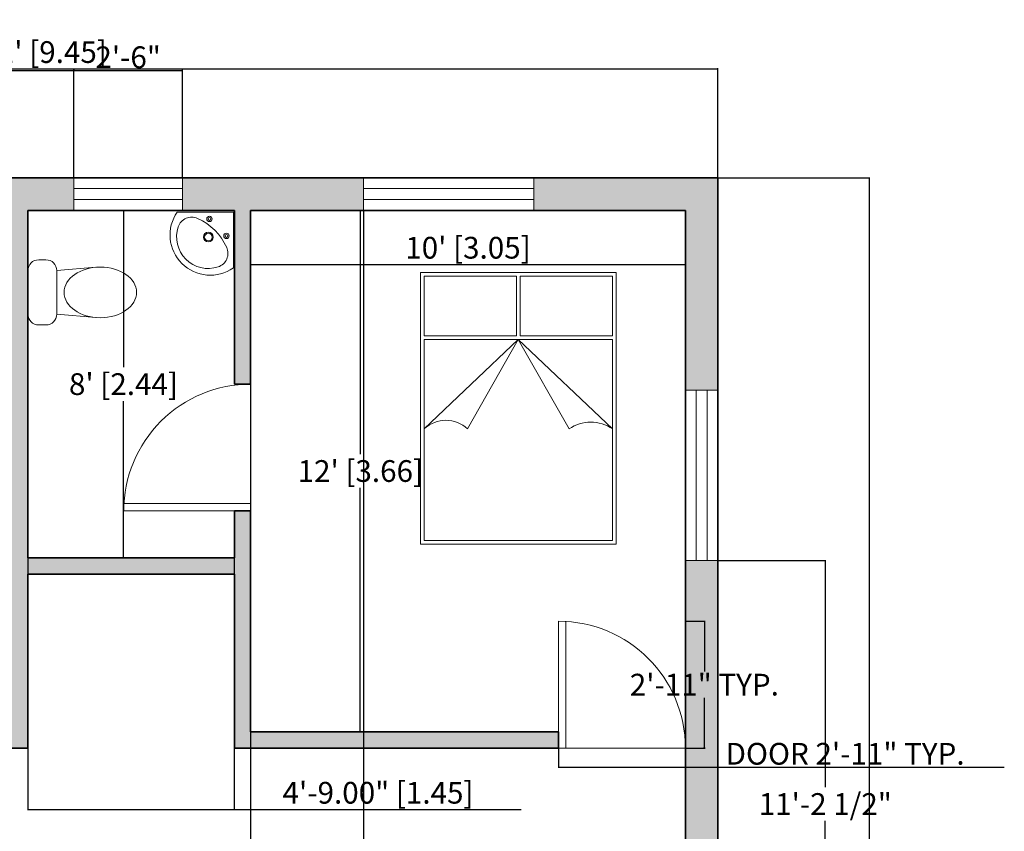
# Model space of a CAD drawing. Units: inches. Extents: x 2322 to 2932, y 142 to 762.
# Tile 7 of 7: x 2609 to 2881, y 538 to 762. Entities that reach past the tile are written whole.
import ezdxf

# ---------------------------------------------------------------- set-up
doc = ezdxf.new("R2010")
doc.units = ezdxf.units.IN
doc.header["$MEASUREMENT"] = 0
for name, color, linetype, lineweight in [('A-ANNO-DIMS', 2, 'Continuous', 18), ('A-DOOR', 3, 'Continuous', 18), ('A-FLOR-FIXT', 9, 'Continuous', 18), ('A-GLAZ', 4, 'Continuous', 18), ('A-WALL', 7, 'Continuous', 35)]:
    doc.layers.add(name, color=color, linetype=linetype, lineweight=lineweight)
doc.layers.add('A-WALL-PATT', color=40, linetype='Continuous', lineweight=13, true_color=0xf8d731)
doc.layers.add('Furniture', color=7, linetype='Continuous', lineweight=15, true_color=0xffffff)
doc.styles.get("Standard").update_dxf_attribs({"font": 'italic8.shx'})
doc.dimstyles.get("Standard").update_dxf_attribs({"dimtxt": 6, "dimasz": 0.15, "dimexe": 0.18, "dimexo": 0.0625, "dimgap": 0.09, "dimtad": 1, "dimtih": 1, "dimtoh": 1, "dimzin": 0, "dimdsep": 46, "dimlunit": 3, "dimtxsty": 'Standard', "dimblk": 'CLOSEDBLANK', "dimcen": 0.09, "dimclrd": 3, "dimclre": 1, "dimclrt": 6, "dimadec": 0, "dimazin": 0, "dimtfac": 1, "dimtofl": 0, "dimtmove": 0, "dimatfit": 3, "dimldrblk": 'DOT', "dimfxl": 1, "dimtolj": 1, "dimtzin": 0, "dimarcsym": 0})

# ---------------------------------------------------------------- blocks, each defined once
blk = doc.blocks.new('_ClosedBlank')
at = {"color": 0, "linetype": 'ByBlock', "lineweight": -2}
for p, q in [((-1, 0.2), (0, 0)), ((-1, 0.2), (-1, -0.2)), ((0, 0), (-1, -0.2))]:
    blk.add_line(p, q, dxfattribs=at)
blk = doc.blocks.new('*D3')
at = {"layer": 'A-ANNO-DIMS', "color": 0, "lineweight": -2, "transparency": 16777216}
for p, q in [((2802.13, 718.82), (2844.02, 718.82)), ((2843.84, 718.67), (2843.84, 451.98)), ((2843.84, 175.97), (2843.84, 442.66)), ((2802.13, 175.82), (2844.02, 175.82))]:
    blk.add_line(p, q, dxfattribs=at)
at = {"layer": 'Defpoints', "color": 0, "transparency": 16777216}
for p in [(2802.06, 718.82), (2802.06, 175.82), (2843.84, 175.82)]:
    blk.add_point(p, dxfattribs=at)
at = {"layer": 'A-ANNO-DIMS', "color": 0, "lineweight": -2, "transparency": 16777216, "xscale": 0.15, "yscale": 0.15, "zscale": 0.15}
for p, rotation in [((2843.84, 718.82), 90), ((2843.84, 175.82), 270)]:
    blk.add_blockref('_ClosedBlank', p, dxfattribs=dict(at, rotation=rotation))
at = {"layer": 'A-ANNO-DIMS', "color": 0, "transparency": 16777216, "insert": (2843.84, 447.32), "char_height": 6, "attachment_point": 5}
blk.add_mtext('\\A1;45\'-3.00" [13.79]', dxfattribs=at)
blk = doc.blocks.new('_Dot')
at = {"color": 0, "linetype": 'ByBlock', "lineweight": -2}
blk.add_line((-0.5, 0), (-1, 0), dxfattribs=at)
at = {"color": 0, "linetype": 'ByBlock', "const_width": 0.5}
blk.add_lwpolyline([(-0.25, 0, 1), (0.25, 0, 1)], format="xyb", close=True, dxfattribs=at)
blk = doc.blocks.new('*D7')
at = {"layer": 'A-ANNO-DIMS', "color": 0, "lineweight": -2, "transparency": 16777216}
for p, q in [((2430.06, 718.88), (2430.06, 749.05)), ((2430.21, 748.87), (2801.91, 748.87)), ((2802.06, 718.88), (2802.06, 749.05))]:
    blk.add_line(p, q, dxfattribs=at)
at = {"layer": 'Defpoints', "color": 0, "transparency": 16777216}
for p in [(2802.06, 748.87), (2430.06, 718.82), (2802.06, 718.82)]:
    blk.add_point(p, dxfattribs=at)
at = {"layer": 'A-ANNO-DIMS', "color": 0, "lineweight": -2, "transparency": 16777216, "xscale": 0.15, "yscale": 0.15, "zscale": 0.15, "rotation": 180}
blk.add_blockref('_ClosedBlank', (2430.06, 748.87), dxfattribs=at)
at = {"layer": 'A-ANNO-DIMS', "color": 0, "lineweight": -2, "transparency": 16777216, "xscale": 0.15, "yscale": 0.15, "zscale": 0.15}
blk.add_blockref('_ClosedBlank', (2802.06, 748.87), dxfattribs=at)
at = {"layer": 'A-ANNO-DIMS', "color": 0, "transparency": 16777216, "insert": (2616.06, 753.53), "char_height": 6, "attachment_point": 5}
blk.add_mtext("\\A1;31' [9.45]", dxfattribs=at)
blk = doc.blocks.new('*D11')
at = {"layer": 'A-ANNO-DIMS', "color": 0, "lineweight": -2, "transparency": 16777216}
for p, q in [((2673.06, 685.88), (2673.06, 695.01)), ((2673.21, 694.83), (2792.91, 694.83)), ((2793.06, 685.88), (2793.06, 695.01))]:
    blk.add_line(p, q, dxfattribs=at)
at = {"layer": 'Defpoints', "color": 0, "transparency": 16777216}
for p in [(2793.06, 694.83), (2673.06, 685.82), (2793.06, 685.82)]:
    blk.add_point(p, dxfattribs=at)
at = {"layer": 'A-ANNO-DIMS', "color": 0, "lineweight": -2, "transparency": 16777216, "xscale": 0.15, "yscale": 0.15, "zscale": 0.15, "rotation": 180}
blk.add_blockref('_ClosedBlank', (2673.06, 694.83), dxfattribs=at)
at = {"layer": 'A-ANNO-DIMS', "color": 0, "lineweight": -2, "transparency": 16777216, "xscale": 0.15, "yscale": 0.15, "zscale": 0.15}
blk.add_blockref('_ClosedBlank', (2793.06, 694.83), dxfattribs=at)
at = {"layer": 'A-ANNO-DIMS', "color": 0, "transparency": 16777216, "insert": (2733.06, 699.49), "char_height": 6, "attachment_point": 5}
blk.add_mtext("\\A1;10' [3.05]", dxfattribs=at)
blk = doc.blocks.new('*D12')
at = {"layer": 'A-ANNO-DIMS', "color": 0, "lineweight": -2, "transparency": 16777216}
for p, q in [((2701.93, 709.82), (2703.52, 709.82)), ((2703.34, 709.67), (2703.34, 642.48)), ((2703.34, 565.97), (2703.34, 633.16)), ((2701.93, 565.82), (2703.52, 565.82))]:
    blk.add_line(p, q, dxfattribs=at)
at = {"layer": 'Defpoints', "color": 0, "transparency": 16777216}
for p in [(2701.87, 709.82), (2701.87, 565.82), (2703.34, 565.82)]:
    blk.add_point(p, dxfattribs=at)
at = {"layer": 'A-ANNO-DIMS', "color": 0, "lineweight": -2, "transparency": 16777216, "xscale": 0.15, "yscale": 0.15, "zscale": 0.15}
for p, rotation in [((2703.34, 709.82), 90), ((2703.34, 565.82), 270)]:
    blk.add_blockref('_ClosedBlank', p, dxfattribs=dict(at, rotation=rotation))
at = {"layer": 'A-ANNO-DIMS', "color": 0, "transparency": 16777216, "insert": (2703.34, 637.82), "char_height": 6, "attachment_point": 5}
blk.add_mtext("\\A1;12' [3.66]", dxfattribs=at)
blk = doc.blocks.new('*D13')
at = {"layer": 'A-ANNO-DIMS', "color": 0, "lineweight": -2, "transparency": 16777216}
for p, q in [((2627.63, 709.82), (2638.14, 709.82)), ((2637.96, 709.67), (2637.96, 666.48)), ((2637.96, 613.97), (2637.96, 657.16)), ((2627.63, 613.82), (2638.14, 613.82))]:
    blk.add_line(p, q, dxfattribs=at)
at = {"layer": 'Defpoints', "color": 0, "transparency": 16777216}
for p in [(2627.57, 709.82), (2637.96, 709.82), (2627.57, 613.82)]:
    blk.add_point(p, dxfattribs=at)
at = {"layer": 'A-ANNO-DIMS', "color": 0, "lineweight": -2, "transparency": 16777216, "xscale": 0.15, "yscale": 0.15, "zscale": 0.15}
for p, rotation in [((2637.96, 709.82), 90), ((2637.96, 613.82), 270)]:
    blk.add_blockref('_ClosedBlank', p, dxfattribs=dict(at, rotation=rotation))
at = {"layer": 'A-ANNO-DIMS', "color": 0, "transparency": 16777216, "insert": (2637.96, 661.82), "char_height": 6, "attachment_point": 5}
blk.add_mtext("\\A1;8' [2.44]", dxfattribs=at)
blk = doc.blocks.new('*D18')
at = {"layer": 'A-ANNO-DIMS', "color": 0, "lineweight": -2, "transparency": 16777216}
for p, q in [((2611.56, 621.53), (2611.56, 544.12)), ((2668.56, 620.26), (2668.56, 544.12)), ((2611.71, 544.3), (2668.41, 544.3)), ((2668.56, 544.3), (2747.75, 544.3))]:
    blk.add_line(p, q, dxfattribs=at)
at = {"layer": 'Defpoints', "color": 0, "transparency": 16777216}
for p in [(2611.56, 621.59), (2668.56, 620.32), (2668.56, 544.3)]:
    blk.add_point(p, dxfattribs=at)
at = {"layer": 'A-ANNO-DIMS', "color": 0, "lineweight": -2, "transparency": 16777216, "xscale": 0.15, "yscale": 0.15, "zscale": 0.15, "rotation": 180}
blk.add_blockref('_ClosedBlank', (2611.56, 544.3), dxfattribs=at)
at = {"layer": 'A-ANNO-DIMS', "color": 0, "lineweight": -2, "transparency": 16777216, "xscale": 0.15, "yscale": 0.15, "zscale": 0.15}
blk.add_blockref('_ClosedBlank', (2668.56, 544.3), dxfattribs=at)
at = {"layer": 'A-ANNO-DIMS', "color": 0, "transparency": 16777216, "insert": (2708.23, 548.96), "char_height": 6, "attachment_point": 5}
blk.add_mtext('\\A1;4\'-9.00" [1.45]', dxfattribs=at)
blk = doc.blocks.new('DOOR-SWING-35')
for p, q in [((0, 35), (0, 0)), ((2, 35), (2, 0)), ((0, 0), (35, 0))]:
    blk.add_line(p, q)
blk.add_arc((0, 0), 35, 0, 90)
blk = doc.blocks.new('WINDOW-47X9')
for p, q in [((47, 9), (0, 9)), ((0, 9), (0, 0)), ((47, 0), (47, 9)), ((0, 6), (47, 6)), ((0, 3), (47, 3)), ((0, 0), (47, 0))]:
    blk.add_line(p, q)
blk = doc.blocks.new('WC-TANK')
for p, q in [((3, 18), (5, 18)), ((0, 3), (0, 15)), ((8, 15), (18.75, 15.95)), ((8, 15), (8, 3)), ((8, 3), (18.75, 2.05)), ((5, 0), (3, 0))]:
    blk.add_line(p, q)
for centre, start, end in [((3, 15), 90, 180), ((5, 15), 0, 90), ((3, 3), 180, 270), ((5, 3), 270, 0)]:
    blk.add_arc(centre, 3, start, end)
blk.add_ellipse((20, 9), major_axis=(10, 0), ratio=0.7)
blk = doc.blocks.new('BED-DOUBLE')
for p, q in [((0, 75), (54, 75)), ((0, 0), (0, 75)), ((1, 74), (26.5, 74)), ((1, 57.55), (1, 74)), ((26.5, 57.55), (26.5, 74)), ((27.5, 74), (53, 74)), ((27.5, 57.55), (27.5, 74)), ((53, 74), (53, 57.55)), ((54, 75), (54, 0)), ((1, 57.55), (26.5, 57.55)), ((27.5, 57.55), (53, 57.55)), ((1, 1), (1, 56.55)), ((1, 56.55), (53, 56.55)), ((27, 56.55), (1, 31.82)), ((13, 31.82), (27, 56.55)), ((27, 56.55), (53, 31.82)), ((41, 31.82), (27, 56.55)), ((53, 56.55), (53, 1)), ((54, 0), (0, 0)), ((53, 1), (1, 1))]:
    blk.add_line(p, q)
for centre, radius, start, end in [((7, 25.51), 8.71, 46.4371, 133.5629), ((47, 23.41), 10.33, 54.4852, 125.5148)]:
    blk.add_arc(centre, radius, start, end)
blk = doc.blocks.new('*D34')
at = {"layer": 'A-ANNO-DIMS', "color": 1, "lineweight": -2, "transparency": 16777216}
for p, q in [((2758.06, 561.26), (2758.06, 555.89)), ((2793.06, 561.26), (2793.06, 555.89))]:
    blk.add_line(p, q, dxfattribs=at)
at = {"layer": 'A-ANNO-DIMS', "color": 3, "lineweight": -2, "transparency": 16777216}
for p, q in [((2758.21, 556.07), (2792.91, 556.07)), ((2793.06, 556.07), (2881.11, 556.07))]:
    blk.add_line(p, q, dxfattribs=at)
at = {"layer": 'Defpoints', "color": 0, "transparency": 16777216}
for p in [(2758.06, 561.32), (2793.06, 561.32), (2793.06, 556.07)]:
    blk.add_point(p, dxfattribs=at)
at = {"layer": 'A-ANNO-DIMS', "color": 3, "lineweight": -2, "transparency": 16777216, "xscale": 0.15, "yscale": 0.15, "zscale": 0.15, "rotation": 180}
blk.add_blockref('_ClosedBlank', (2758.06, 556.07), dxfattribs=at)
at = {"layer": 'A-ANNO-DIMS', "color": 3, "lineweight": -2, "transparency": 16777216, "xscale": 0.15, "yscale": 0.15, "zscale": 0.15}
blk.add_blockref('_ClosedBlank', (2793.06, 556.07), dxfattribs=at)
at = {"layer": 'A-ANNO-DIMS', "color": 6, "transparency": 16777216, "insert": (2837.16, 559.73), "char_height": 6, "attachment_point": 5}
blk.add_mtext('\\A1;DOOR 2\'-11" TYP.', dxfattribs=at)
blk = doc.blocks.new('*D35')
at = {"layer": 'A-ANNO-DIMS', "color": 1, "lineweight": -2, "transparency": 16777216}
for p, q in [((2793.13, 596.32), (2798.49, 596.32)), ((2793.13, 561.32), (2798.49, 561.32))]:
    blk.add_line(p, q, dxfattribs=at)
at = {"layer": 'A-ANNO-DIMS', "color": 3, "lineweight": -2, "transparency": 16777216}
for p, q in [((2798.31, 596.17), (2798.31, 582.48)), ((2798.31, 561.47), (2798.31, 575.16))]:
    blk.add_line(p, q, dxfattribs=at)
at = {"layer": 'Defpoints', "color": 0, "transparency": 16777216}
for p in [(2793.06, 596.32), (2798.31, 596.32), (2793.06, 561.32)]:
    blk.add_point(p, dxfattribs=at)
at = {"layer": 'A-ANNO-DIMS', "color": 3, "lineweight": -2, "transparency": 16777216, "xscale": 0.15, "yscale": 0.15, "zscale": 0.15}
for p, rotation in [((2798.31, 596.32), 90), ((2798.31, 561.32), 270)]:
    blk.add_blockref('_ClosedBlank', p, dxfattribs=dict(at, rotation=rotation))
at = {"layer": 'A-ANNO-DIMS', "color": 6, "transparency": 16777216, "insert": (2798.31, 578.82), "char_height": 6, "attachment_point": 5}
blk.add_mtext('\\A1;2\'-11" TYP.', dxfattribs=at)
blk = doc.blocks.new('*D52')
at = {"layer": 'A-ANNO-DIMS', "color": 1, "lineweight": -2, "transparency": 16777216}
for p, q in [((2538.1, 718.88), (2538.1, 748.62)), ((2624.25, 718.88), (2624.25, 748.62))]:
    blk.add_line(p, q, dxfattribs=at)
at = {"layer": 'A-ANNO-DIMS', "color": 3, "lineweight": -2, "transparency": 16777216}
blk.add_line((2538.25, 748.44), (2624.1, 748.44), dxfattribs=at)
at = {"layer": 'Defpoints', "color": 0, "transparency": 16777216}
for p in [(2624.25, 748.44), (2538.1, 718.82), (2624.25, 718.82)]:
    blk.add_point(p, dxfattribs=at)
at = {"layer": 'A-ANNO-DIMS', "color": 3, "lineweight": -2, "transparency": 16777216, "xscale": 0.15, "yscale": 0.15, "zscale": 0.15, "rotation": 180}
blk.add_blockref('_ClosedBlank', (2538.1, 748.44), dxfattribs=at)
at = {"layer": 'A-ANNO-DIMS', "color": 3, "lineweight": -2, "transparency": 16777216, "xscale": 0.15, "yscale": 0.15, "zscale": 0.15}
blk.add_blockref('_ClosedBlank', (2624.25, 748.44), dxfattribs=at)
at = {"layer": 'A-ANNO-DIMS', "color": 6, "transparency": 16777216, "insert": (2581.17, 752.1), "char_height": 6, "attachment_point": 5}
blk.add_mtext('\\A1;7\'-2"', dxfattribs=at)
blk = doc.blocks.new('*D53')
at = {"layer": 'A-ANNO-DIMS', "color": 1, "lineweight": -2, "transparency": 16777216}
for p, q in [((2624.25, 718.88), (2624.25, 748.62)), ((2654.25, 718.88), (2654.25, 748.62))]:
    blk.add_line(p, q, dxfattribs=at)
at = {"layer": 'A-ANNO-DIMS', "color": 3, "lineweight": -2, "transparency": 16777216}
blk.add_line((2624.4, 748.44), (2654.1, 748.44), dxfattribs=at)
at = {"layer": 'Defpoints', "color": 0, "transparency": 16777216}
for p in [(2654.25, 748.44), (2624.25, 718.82), (2654.25, 718.82)]:
    blk.add_point(p, dxfattribs=at)
at = {"layer": 'A-ANNO-DIMS', "color": 3, "lineweight": -2, "transparency": 16777216, "xscale": 0.15, "yscale": 0.15, "zscale": 0.15, "rotation": 180}
blk.add_blockref('_ClosedBlank', (2624.25, 748.44), dxfattribs=at)
at = {"layer": 'A-ANNO-DIMS', "color": 3, "lineweight": -2, "transparency": 16777216, "xscale": 0.15, "yscale": 0.15, "zscale": 0.15}
blk.add_blockref('_ClosedBlank', (2654.25, 748.44), dxfattribs=at)
at = {"layer": 'A-ANNO-DIMS', "color": 6, "transparency": 16777216, "insert": (2639.25, 752.1), "char_height": 6, "attachment_point": 5}
blk.add_mtext('\\A1;2\'-6"', dxfattribs=at)
blk = doc.blocks.new('*D54')
at = {"layer": 'A-ANNO-DIMS', "color": 1, "lineweight": -2, "transparency": 16777216}
for p, q in [((2673.06, 709.76), (2673.06, 146.01)), ((2704.23, 709.76), (2704.23, 146.01))]:
    blk.add_line(p, q, dxfattribs=at)
at = {"layer": 'A-ANNO-DIMS', "color": 3, "lineweight": -2, "transparency": 16777216}
blk.add_line((2673.21, 146.19), (2704.08, 146.19), dxfattribs=at)
at = {"layer": 'Defpoints', "color": 0, "transparency": 16777216}
for p in [(2673.06, 709.82), (2704.23, 709.82), (2704.23, 146.19)]:
    blk.add_point(p, dxfattribs=at)
at = {"layer": 'A-ANNO-DIMS', "color": 3, "lineweight": -2, "transparency": 16777216, "xscale": 0.15, "yscale": 0.15, "zscale": 0.15, "rotation": 180}
blk.add_blockref('_ClosedBlank', (2673.06, 146.19), dxfattribs=at)
at = {"layer": 'A-ANNO-DIMS', "color": 3, "lineweight": -2, "transparency": 16777216, "xscale": 0.15, "yscale": 0.15, "zscale": 0.15}
blk.add_blockref('_ClosedBlank', (2704.23, 146.19), dxfattribs=at)
at = {"layer": 'A-ANNO-DIMS', "color": 6, "transparency": 16777216, "insert": (2688.65, 149.85), "char_height": 6, "attachment_point": 5}
blk.add_mtext('\\A1;2\'-7"', dxfattribs=at)
blk = doc.blocks.new('*D64')
at = {"layer": 'A-ANNO-DIMS', "color": 1, "lineweight": -2, "transparency": 16777216}
for p, q in [((2802.13, 613.14), (2831.87, 613.14)), ((2802.13, 478.57), (2831.87, 478.57))]:
    blk.add_line(p, q, dxfattribs=at)
at = {"layer": 'A-ANNO-DIMS', "color": 3, "lineweight": -2, "transparency": 16777216}
for p, q in [((2831.69, 612.99), (2831.69, 550.51)), ((2831.69, 478.72), (2831.69, 541.19))]:
    blk.add_line(p, q, dxfattribs=at)
at = {"layer": 'Defpoints', "color": 0, "transparency": 16777216}
for p in [(2802.06, 613.14), (2831.69, 613.14), (2802.06, 478.57)]:
    blk.add_point(p, dxfattribs=at)
at = {"layer": 'A-ANNO-DIMS', "color": 3, "lineweight": -2, "transparency": 16777216, "xscale": 0.15, "yscale": 0.15, "zscale": 0.15}
for p, rotation in [((2831.69, 613.14), 90), ((2831.69, 478.57), 270)]:
    blk.add_blockref('_ClosedBlank', p, dxfattribs=dict(at, rotation=rotation))
at = {"layer": 'A-ANNO-DIMS', "color": 6, "transparency": 16777216, "insert": (2831.69, 545.85), "char_height": 6, "attachment_point": 5}
blk.add_mtext('\\A1;11\'-2 1/2"', dxfattribs=at)

msp = doc.modelspace()

# ---------------------------------------------------------------- hatches: boundary and pattern name
at = {"layer": 'A-WALL-PATT'}
h = msp.add_hatch(color=256, dxfattribs=at)
h.dxf.hatch_style = 1
h.paths.add_polyline_path([(2439.065, 709.819), (2491.097, 709.819), (2491.097, 718.819), (2430.065, 718.819), (2430.065, 663.548), (2439.065, 663.548)])
h.paths.add_polyline_path([(2704.233, 718.819), (2654.246, 718.819), (2654.246, 709.819), (2668.565, 709.819), (2668.565, 661.819), (2673.065, 661.819), (2673.065, 709.819), (2704.233, 709.819)], flags=17)
h.paths.add_polyline_path([(2624.246, 718.819), (2538.097, 718.819), (2538.097, 709.819), (2607.065, 709.819), (2607.065, 565.819), (2583.065, 565.819), (2583.065, 561.319), (2611.565, 561.319), (2611.565, 609.319), (2668.565, 609.319), (2668.565, 561.319), (2758.065, 561.319), (2758.065, 565.819), (2673.065, 565.819), (2673.065, 626.819), (2668.565, 626.819), (2668.565, 613.819), (2611.565, 613.819), (2611.565, 709.819), (2624.246, 709.819)])
h.paths.add_polyline_path([(2802.065, 718.819), (2751.233, 718.819), (2751.233, 709.819), (2793.065, 709.819), (2793.065, 660.138), (2802.065, 660.138)])
h.paths.add_polyline_path([(2802.065, 613.138), (2793.065, 613.138), (2793.065, 478.568), (2802.065, 478.568)])
h.paths.add_polyline_path([(2439.065, 616.548), (2430.065, 616.548), (2430.065, 551.562), (2439.065, 551.562), (2439.065, 561.319), (2483.455, 561.319), (2483.455, 565.819), (2439.065, 565.819)])
h.paths.add_polyline_path([(2548.065, 565.819), (2518.455, 565.819), (2518.455, 561.319), (2541.065, 561.319), (2541.065, 501.319), (2439.065, 501.319), (2439.065, 516.562), (2430.065, 516.562), (2430.065, 465.181), (2439.065, 465.181), (2439.065, 496.819), (2503.266, 496.819), (2541.065, 496.819), (2541.065, 472.819), (2545.565, 472.819), (2545.565, 561.319), (2548.065, 561.319)])
h.paths.add_polyline_path([(2439.065, 418.181), (2430.065, 418.181), (2430.065, 342.453), (2439.065, 342.453), (2439.065, 367.819), (2602.565, 367.819), (2602.565, 283.756), (2594.693, 283.756), (2594.693, 274.756), (2611.565, 274.756), (2611.565, 501.319), (2580.942, 501.319), (2580.942, 496.819), (2607.065, 496.819), (2607.065, 376.819), (2439.065, 376.819)])
h.paths.add_polyline_path([(2793.057, 530.805), (2793.057, 530.68), (2793.106, 530.68), (2793.106, 530.805)], flags=25)
h.paths.add_polyline_path([(2793.057, 530.808), (2793.057, 530.676), (2793.106, 530.676), (2793.106, 530.808)], flags=9)

# ---------------------------------------------------------------- linework, layer by layer
at = {"layer": 'A-FLOR-FIXT'}
for q in [(2652.815, 709.351), (2668.3, 693.935)]:
    msp.add_line((2668.3, 709.351), q, dxfattribs=at)
for centre, radius in [((2661.705, 707.449), 0.749), ((2661.705, 707.449), 0.394), ((2661.399, 702.45), 1.364), ((2661.399, 702.45), 1.042), ((2666.399, 702.756), 0.749), ((2666.399, 702.756), 0.394)]:
    msp.add_circle(centre, radius, dxfattribs=at)
for centre, radius, start, end in [((2661.902, 702.994), 11.09, 145.02413, 305.23469), ((2656.805, 704.008), 3.937, 65.61574, 161.56511), ((2651.77, 692.902), 16.131, 24.38426, 65.61574), ((2661.359, 702.49), 8.737, 161.56511, 288.43489), ((2662.877, 697.936), 3.937, 288.43489, 24.38426)]:
    msp.add_arc(centre, radius, start, end, dxfattribs=at)
at = {"layer": 'A-GLAZ'}
for p, q in [((2624.246, 718.819), (2654.246, 718.819)), ((2624.246, 709.819), (2624.246, 718.819)), ((2654.246, 718.819), (2654.246, 709.819)), ((2624.246, 715.819), (2654.246, 715.819)), ((2624.246, 712.819), (2654.246, 712.819)), ((2654.246, 709.819), (2624.246, 709.819))]:
    msp.add_line(p, q, dxfattribs=at)
at = {"layer": 'A-WALL'}
for p, q in [((2802.065, 718.819), (2430.065, 718.819)), ((2802.065, 175.819), (2802.065, 718.819)), ((2611.565, 709.819), (2611.565, 613.819)), ((2668.565, 709.819), (2611.565, 709.819)), ((2668.565, 709.819), (2668.565, 661.819)), ((2793.065, 709.819), (2673.065, 709.819)), ((2673.065, 709.819), (2673.065, 661.819)), ((2793.065, 283.756), (2793.065, 709.819)), ((2668.565, 661.819), (2673.065, 661.819)), ((2668.565, 626.819), (2673.065, 626.819)), ((2668.565, 626.819), (2668.565, 613.819)), ((2673.065, 626.819), (2673.065, 565.819)), ((2668.565, 613.819), (2611.565, 613.819)), ((2668.565, 609.319), (2611.565, 609.319)), ((2611.565, 609.319), (2611.565, 561.319)), ((2668.565, 609.319), (2668.565, 561.319)), ((2758.065, 565.819), (2673.065, 565.819)), ((2758.065, 561.319), (2758.065, 565.819)), ((2611.565, 561.319), (2583.065, 561.319)), ((2758.065, 561.319), (2668.565, 561.319))]:
    msp.add_line(p, q, dxfattribs=at)

# ---------------------------------------------------------------- block references
at = {"layer": 'A-DOOR', "rotation": 89.99999999999959}
msp.add_blockref('DOOR-SWING-35', (2673.064, 626.82), dxfattribs=at)
at = {"layer": 'A-DOOR'}
msp.add_blockref('DOOR-SWING-35', (2758.065, 561.319), dxfattribs=at)
at = {"layer": 'A-FLOR-FIXT'}
msp.add_blockref('WC-TANK', (2611.565, 678.157), dxfattribs=at)
at = {"layer": 'A-GLAZ'}
msp.add_blockref('WINDOW-47X9', (2704.233, 709.819), dxfattribs=at)
at = {"layer": 'A-GLAZ', "rotation": 90.0000000000009}
msp.add_blockref('WINDOW-47X9', (2802.064, 613.138), dxfattribs=at)
at = {"layer": 'Furniture'}
msp.add_blockref('BED-DOUBLE', (2719.96, 617.61), dxfattribs=at)

# ---------------------------------------------------------------- dimensions: what is measured, and where the dimension line sits
at = {"layer": 'A-ANNO-DIMS'}
for base, p1, p2, override, picture, middle in [((2802.065, 748.867), (2430.065, 718.819), (2802.065, 718.819), {"dimclrd": 0, "dimclre": 0, "dimclrt": 0}, '*D7', (2616.065, 753.528)), ((2624.246, 748.444), (2538.097, 718.819), (2624.246, 718.819), {"dimdec": 1, "dimlfac": 1, "dimrnd": 0, "dimzin": 1, "dimdsep": 46, "dimlunit": 4, "dimfrac": 2}, '*D52', (2581.172, 752.105)), ((2654.246, 748.444), (2624.246, 718.819), (2654.246, 718.819), {"dimdec": 1, "dimlfac": 1, "dimrnd": 0, "dimzin": 1, "dimdsep": 46, "dimlunit": 4, "dimfrac": 2}, '*D53', (2639.246, 752.105)), ((2704.233, 146.194), (2673.065, 709.819), (2704.233, 709.819), {"dimdec": 1, "dimlfac": 1, "dimrnd": 0, "dimzin": 1, "dimdsep": 46, "dimlunit": 4, "dimfrac": 2}, '*D54', (2688.649, 149.855)), ((2793.065, 694.828), (2673.065, 685.819), (2793.065, 685.819), {"dimclrd": 0, "dimclre": 0, "dimclrt": 0}, '*D11', (2733.065, 699.49)), ((2668.565, 544.299), (2611.565, 621.593), (2668.565, 620.319), {"dimclrd": 0, "dimclre": 0, "dimclrt": 0}, '*D18', (2708.233, 548.961))]:
    dim = msp.add_linear_dim(base=base, p1=p1, p2=p2, dimstyle='Standard', override=override, dxfattribs=at)
    dim.commit()
    dim.dimension.update_dxf_attribs({"geometry": picture, "text_midpoint": middle})
for base, p1, p2, override, picture, middle in [((2843.838, 175.819), (2802.065, 718.819), (2802.065, 175.819), {"dimclrd": 0, "dimclre": 0, "dimclrt": 0}, '*D3', (2843.838, 447.319)), ((2637.956, 709.819), (2627.568, 613.819), (2627.568, 709.819), {"dimclrd": 0, "dimclre": 0, "dimclrt": 0}, '*D13', (2637.956, 661.819)), ((2703.341, 565.819), (2701.87, 709.819), (2701.87, 565.819), {"dimclrd": 0, "dimclre": 0, "dimclrt": 0}, '*D12', (2703.341, 637.819)), ((2831.69, 613.138), (2802.065, 478.568), (2802.065, 613.138), {"dimdec": 1, "dimlfac": 1, "dimrnd": 0, "dimzin": 1, "dimdsep": 46, "dimlunit": 4, "dimfrac": 2}, '*D64', (2831.69, 545.853))]:
    dim = msp.add_linear_dim(base=base, p1=p1, p2=p2, angle=90, dimstyle='Standard', override=override, dxfattribs=at)
    dim.commit()
    dim.dimension.update_dxf_attribs({"geometry": picture, "text_midpoint": middle})
dim = msp.add_linear_dim(base=(2798.315, 596.319), p1=(2793.065, 561.319), p2=(2793.065, 596.319), angle=90, text='<> TYP.', dimstyle='Standard', override={"dimdec": 1, "dimlfac": 1, "dimrnd": 0, "dimzin": 1, "dimdsep": 46, "dimlunit": 4, "dimfrac": 2}, dxfattribs=at)
dim.commit()
dim.dimension.update_dxf_attribs({"geometry": '*D35', "text_midpoint": (2798.315, 578.819)})
dim = msp.add_linear_dim(base=(2793.065, 556.069), p1=(2758.065, 561.319), p2=(2793.065, 561.319), text='DOOR <> TYP.', dimstyle='Standard', override={"dimdec": 1, "dimlfac": 1, "dimrnd": 0, "dimzin": 1, "dimdsep": 46, "dimlunit": 4, "dimfrac": 2}, dxfattribs=at)
dim.commit()
dim.dimension.update_dxf_attribs({"geometry": '*D34', "text_midpoint": (2837.162, 559.73)})

doc.saveas('drawing.dxf')
